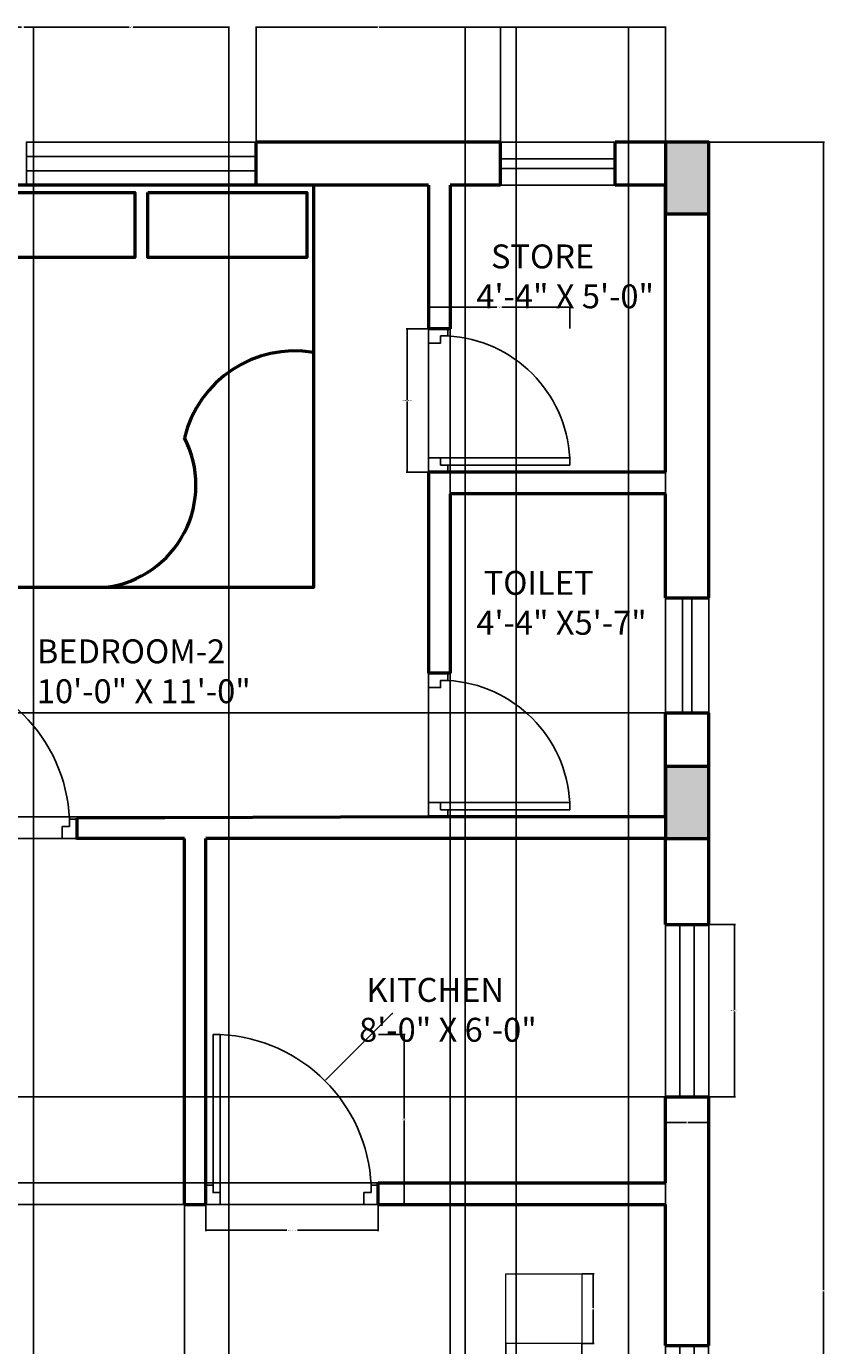
# Model space of a CAD drawing. Units: inches. Extents: x 2480 to 2840, y 795 to 1323.
# Tile 4 of 4: x 2673 to 2840, y 1047 to 1323. Entities that reach past the tile are written whole.
import ezdxf

# ---------------------------------------------------------------- set-up
doc = ezdxf.new("R2010")
doc.units = ezdxf.units.IN
for name, color, linetype, lineweight in [('A-ANNO-DIMS', 2, 'Continuous', 18), ('A-AREA-IDEN', 7, 'Continuous', 25), ('COLUMN', 240, 'Continuous', 50), ('door', 140, 'Continuous', 25), ('Furniture', 9, 'Continuous', 18), ('ventilator', 32, 'Continuous', 25), ('wall', 7, 'Continuous', 50), ('window', 201, 'Continuous', 25)]:
    doc.layers.add(name, color=color, linetype=linetype, lineweight=lineweight)
doc.styles.get("Standard").update_dxf_attribs({"font": 'arial.ttf'})
doc.dimstyles.get("Standard").update_dxf_attribs({"dimtxt": 0.18, "dimasz": 0.18, "dimexe": 0.18, "dimexo": 0.0625, "dimgap": 0.09, "dimtad": 0, "dimtih": 1, "dimtoh": 1, "dimdec": 4, "dimzin": 0, "dimdsep": 46, "dimtxsty": 'Standard', "dimcen": 0.09, "dimadec": 0, "dimazin": 0, "dimtfac": 1, "dimtdec": 4, "dimtofl": 0, "dimtmove": 0, "dimatfit": 3, "dimfxl": 1, "dimtolj": 1, "dimtzin": 0, "dimarcsym": 0})

# ---------------------------------------------------------------- blocks, each defined once
blk = doc.blocks.new('d1')
at = {"layer": 'door'}
blk.add_line((3049.73, 1052.02), (3085.73, 1052.02), dxfattribs=at)
blk.add_lwpolyline([(3051.23, 1054.52), (3052.73, 1054.52), (3052.73, 1087.52), (3051.23, 1087.52)], close=True, dxfattribs=at)
for points in [[(3052.73, 1052.02), (3049.73, 1052.02), (3049.73, 1056.02), (3051.23, 1056.02), (3051.23, 1054.52), (3052.73, 1054.52), (3052.73, 1052.02)], [(3082.73, 1052.02), (3085.73, 1052.02), (3085.73, 1056.02), (3084.23, 1056.02), (3084.23, 1054.52), (3082.73, 1054.52), (3082.73, 1052.02)]]:
    blk.add_lwpolyline(points, dxfattribs=at)
blk.add_arc((3051.23, 1054.52), 33.03, 2.6026, 87.3974, dxfattribs=at)
blk = doc.blocks.new('w2')
at = {"layer": 'window'}
for p, q in [((2880.46, 1137.77), (2880.46, 1101.77)), ((2883.46, 1137.77), (2883.46, 1101.77))]:
    blk.add_line(p, q, dxfattribs=at)
blk.add_lwpolyline([(2877.46, 1101.77), (2886.46, 1101.77), (2886.46, 1137.77), (2877.46, 1137.77)], close=True, dxfattribs=at)
blk = doc.blocks.new('v')
at = {"layer": 'ventilator'}
for p, q in [((2939.68, 1237.47), (2939.68, 1213.47)), ((2941.68, 1237.47), (2941.68, 1213.47))]:
    blk.add_line(p, q, dxfattribs=at)
blk.add_lwpolyline([(2936.18, 1213.47), (2945.18, 1213.47), (2945.18, 1237.47), (2936.18, 1237.47)], close=True, dxfattribs=at)
blk = doc.blocks.new('w1')
at = {"layer": 'window'}
for p, q in [((2922.2, 1100.57), (2922.2, 1052.57)), ((2925.2, 1100.57), (2925.2, 1052.57))]:
    blk.add_line(p, q, dxfattribs=at)
blk.add_lwpolyline([(2919.2, 1052.57), (2928.2, 1052.57), (2928.2, 1100.57), (2919.2, 1100.57)], close=True, dxfattribs=at)
blk = doc.blocks.new('d2')
at = {"layer": 'door'}
blk.add_line((3049.73, 993.24), (3079.73, 993.24), dxfattribs=at)
blk.add_lwpolyline([(3051.23, 995.74), (3052.73, 995.74), (3052.73, 1022.74), (3051.23, 1022.74)], close=True, dxfattribs=at)
for points in [[(3052.73, 993.24), (3049.73, 993.24), (3049.73, 997.24), (3051.23, 997.24), (3051.23, 995.74), (3052.73, 995.74), (3052.73, 993.24)], [(3076.73, 993.24), (3079.73, 993.24), (3079.73, 997.24), (3078.23, 997.24), (3078.23, 995.74), (3076.73, 995.74), (3076.73, 993.24)]]:
    blk.add_lwpolyline(points, dxfattribs=at)
blk.add_arc((3051.23, 995.74), 27.04, 3.1798, 86.8202, dxfattribs=at)
blk = doc.blocks.new('BED')
at = {"layer": 'wall'}
for points in [[(3037.98, 1220.47), (3109.98, 1220.47), (3109.98, 1304.47), (3037.98, 1304.47)], [(3039.4, 1302.95), (3072.6, 1302.95), (3072.6, 1289.33), (3039.4, 1289.33)], [(3075.32, 1302.95), (3108.52, 1302.95), (3108.52, 1289.33), (3075.32, 1289.33)]]:
    blk.add_lwpolyline(points, close=True, dxfattribs=at)
for centre, radius, start, end in [((3106.11, 1246.04), 23.81, 80.6483, 166.366), ((3063.91, 1241.76), 21.48, 277.4854, 27.4236)]:
    blk.add_arc(centre, radius, start, end, dxfattribs=at)
blk = doc.blocks.new('C')
at = {"layer": 'COLUMN'}
h = blk.add_hatch(color=256, dxfattribs=at)
h.dxf.hatch_style = 1
h.paths.add_polyline_path([(3016.24, 1218.72), (3031.24, 1218.72), (3031.24, 1227.72), (3016.24, 1227.72)])
blk.add_lwpolyline([(3016.24, 1218.72), (3031.24, 1218.72), (3031.24, 1227.72), (3016.24, 1227.72)], close=True, dxfattribs=at)
blk = doc.blocks.new('CHAIR-DINING')
blk.add_lwpolyline([(15.88, 0), (0, 0), (0, 14.61), (15.88, 14.61)], close=True)
blk = doc.blocks.new('*D14')
at = {"layer": 'A-ANNO-DIMS', "color": 0, "lineweight": -2, "transparency": 16777216}
for p, q in [((2816.02, 1135.24), (2821.53, 1135.24)), ((2821.35, 1135.06), (2821.35, 1117.42)), ((2821.35, 1099.42), (2821.35, 1117.06)), ((2816.02, 1099.24), (2821.53, 1099.24))]:
    blk.add_line(p, q, dxfattribs=at)
at = {"layer": 'A-ANNO-DIMS', "color": 0, "transparency": 16777216}
for points in [[(2821.32, 1135.06), (2821.38, 1135.06), (2821.35, 1135.24)], [(2821.32, 1099.42), (2821.38, 1099.42), (2821.35, 1099.24)]]:
    blk.add_solid(points, dxfattribs=at)
at = {"layer": 'Defpoints', "color": 0, "transparency": 16777216}
for p in [(2815.95, 1135.24), (2821.35, 1135.24), (2815.95, 1099.24)]:
    blk.add_point(p, dxfattribs=at)
at = {"layer": 'A-ANNO-DIMS', "color": 0, "transparency": 16777216, "insert": (2821.35, 1117.24), "char_height": 0.18, "attachment_point": 5}
blk.add_mtext('\\A1;WINDOW W2 36', dxfattribs=at)
blk = doc.blocks.new('*D15')
at = {"layer": 'A-ANNO-DIMS', "color": 0, "lineweight": -2, "transparency": 16777216}
for p, q in [((2806.95, 1099.18), (2806.95, 1093.66)), ((2815.95, 1099.18), (2815.95, 1093.66)), ((2807.13, 1093.84), (2811.3, 1093.84)), ((2815.77, 1093.84), (2811.6, 1093.84))]:
    blk.add_line(p, q, dxfattribs=at)
at = {"layer": 'A-ANNO-DIMS', "color": 0, "transparency": 16777216}
for points in [[(2807.13, 1093.87), (2807.13, 1093.81), (2806.95, 1093.84)], [(2815.77, 1093.87), (2815.77, 1093.81), (2815.95, 1093.84)]]:
    blk.add_solid(points, dxfattribs=at)
at = {"layer": 'Defpoints', "color": 0, "transparency": 16777216}
for p in [(2806.95, 1099.24), (2815.95, 1099.24), (2815.95, 1093.84)]:
    blk.add_point(p, dxfattribs=at)
at = {"layer": 'A-ANNO-DIMS', "color": 0, "transparency": 16777216, "insert": (2811.45, 1093.84), "char_height": 0.18, "attachment_point": 5}
blk.add_mtext('\\A1;9', dxfattribs=at)
blk = doc.blocks.new('*D18')
at = {"layer": 'A-ANNO-DIMS', "color": 0, "lineweight": -2, "transparency": 16777216}
for p, q in [((2710.95, 1076.68), (2710.95, 1071.16)), ((2746.95, 1076.68), (2746.95, 1071.16)), ((2711.13, 1071.34), (2727.82, 1071.34)), ((2746.77, 1071.34), (2730.08, 1071.34))]:
    blk.add_line(p, q, dxfattribs=at)
at = {"layer": 'A-ANNO-DIMS', "color": 0, "transparency": 16777216}
for points in [[(2711.13, 1071.37), (2711.13, 1071.31), (2710.95, 1071.34)], [(2746.77, 1071.37), (2746.77, 1071.31), (2746.95, 1071.34)]]:
    blk.add_solid(points, dxfattribs=at)
at = {"layer": 'Defpoints', "color": 0, "transparency": 16777216}
for p in [(2710.95, 1076.74), (2746.95, 1076.74), (2746.95, 1071.34)]:
    blk.add_point(p, dxfattribs=at)
at = {"layer": 'A-ANNO-DIMS', "color": 0, "transparency": 16777216, "insert": (2728.95, 1071.34), "char_height": 0.18, "attachment_point": 5}
blk.add_mtext('\\A1;DOOR D1 36 TYP.', dxfattribs=at)
blk = doc.blocks.new('*D19')
at = {"layer": 'A-ANNO-DIMS', "color": 0, "lineweight": -2, "transparency": 16777216}
for p, q in [((2747.02, 1112.24), (2752.53, 1112.24)), ((2752.35, 1112.06), (2752.35, 1094.67)), ((2752.35, 1076.92), (2752.35, 1094.31)), ((2747.02, 1076.74), (2752.53, 1076.74))]:
    blk.add_line(p, q, dxfattribs=at)
at = {"layer": 'A-ANNO-DIMS', "color": 0, "transparency": 16777216}
for points in [[(2752.32, 1112.06), (2752.38, 1112.06), (2752.35, 1112.24)], [(2752.32, 1076.92), (2752.38, 1076.92), (2752.35, 1076.74)]]:
    blk.add_solid(points, dxfattribs=at)
at = {"layer": 'Defpoints', "color": 0, "transparency": 16777216}
for p in [(2746.95, 1112.24), (2752.35, 1112.24), (2746.95, 1076.74)]:
    blk.add_point(p, dxfattribs=at)
at = {"layer": 'A-ANNO-DIMS', "color": 0, "transparency": 16777216, "insert": (2752.35, 1094.49), "char_height": 0.18, "attachment_point": 5}
blk.add_mtext('\\A1;36 TYP.', dxfattribs=at)
blk = doc.blocks.new('*D20')
at = {"layer": 'A-ANNO-DIMS', "color": 0, "lineweight": -2, "transparency": 16777216}
for p, q in [((2757.39, 1259.74), (2752.77, 1259.74)), ((2752.95, 1259.56), (2752.95, 1244.92)), ((2752.95, 1229.92), (2752.95, 1244.56)), ((2757.39, 1229.74), (2752.77, 1229.74))]:
    blk.add_line(p, q, dxfattribs=at)
at = {"layer": 'A-ANNO-DIMS', "color": 0, "transparency": 16777216}
for points in [[(2752.92, 1259.56), (2752.98, 1259.56), (2752.95, 1259.74)], [(2752.92, 1229.92), (2752.98, 1229.92), (2752.95, 1229.74)]]:
    blk.add_solid(points, dxfattribs=at)
at = {"layer": 'Defpoints', "color": 0, "transparency": 16777216}
for p in [(2752.95, 1259.74), (2757.45, 1259.74), (2757.45, 1229.74)]:
    blk.add_point(p, dxfattribs=at)
at = {"layer": 'A-ANNO-DIMS', "color": 0, "transparency": 16777216, "insert": (2752.95, 1244.74), "char_height": 0.18, "attachment_point": 5}
blk.add_mtext('\\A1;DOOR D2 30 TYP.', dxfattribs=at)
blk = doc.blocks.new('*D21')
at = {"layer": 'A-ANNO-DIMS', "color": 0, "lineweight": -2, "transparency": 16777216}
for p, q in [((2757.45, 1259.8), (2757.45, 1264.42)), ((2757.63, 1264.24), (2771.68, 1264.24)), ((2786.77, 1264.24), (2772.73, 1264.24)), ((2786.95, 1259.8), (2786.95, 1264.42))]:
    blk.add_line(p, q, dxfattribs=at)
at = {"layer": 'A-ANNO-DIMS', "color": 0, "transparency": 16777216}
for points in [[(2757.63, 1264.27), (2757.63, 1264.21), (2757.45, 1264.24)], [(2786.77, 1264.27), (2786.77, 1264.21), (2786.95, 1264.24)]]:
    blk.add_solid(points, dxfattribs=at)
at = {"layer": 'Defpoints', "color": 0, "transparency": 16777216}
for p in [(2786.95, 1264.24), (2757.45, 1259.74), (2786.95, 1259.74)]:
    blk.add_point(p, dxfattribs=at)
at = {"layer": 'A-ANNO-DIMS', "color": 0, "transparency": 16777216, "insert": (2772.2, 1264.24), "char_height": 0.18, "attachment_point": 5}
blk.add_mtext('\\A1;30 TYP.', dxfattribs=at)
blk = doc.blocks.new('*D26')
at = {"layer": 'A-ANNO-DIMS', "color": 0, "lineweight": -2, "transparency": 16777216}
for p, q in [((2773.57, 1047.6), (2773.57, 1045.1)), ((2773.75, 1045.28), (2780.09, 1045.28)), ((2789.27, 1045.28), (2782.94, 1045.28)), ((2789.45, 1047.6), (2789.45, 1045.1))]:
    blk.add_line(p, q, dxfattribs=at)
at = {"layer": 'A-ANNO-DIMS', "color": 0, "transparency": 16777216}
for points in [[(2773.75, 1045.31), (2773.75, 1045.25), (2773.57, 1045.28)], [(2789.27, 1045.31), (2789.27, 1045.25), (2789.45, 1045.28)]]:
    blk.add_solid(points, dxfattribs=at)
at = {"layer": 'Defpoints', "color": 0, "transparency": 16777216}
for p in [(2773.57, 1047.66), (2789.45, 1047.66), (2789.45, 1045.28)]:
    blk.add_point(p, dxfattribs=at)
at = {"layer": 'A-ANNO-DIMS', "color": 0, "transparency": 16777216, "insert": (2781.51, 1045.28), "char_height": 0.18, "attachment_point": 5}
blk.add_mtext('\\A1;DINING CHAIR 16 TYP.', dxfattribs=at)
blk = doc.blocks.new('*D27')
at = {"layer": 'A-ANNO-DIMS', "color": 0, "lineweight": -2, "transparency": 16777216}
for p, q in [((2789.52, 1062.27), (2792.02, 1062.27)), ((2791.84, 1062.09), (2791.84, 1055.15)), ((2791.84, 1047.84), (2791.84, 1054.78)), ((2789.52, 1047.66), (2792.02, 1047.66))]:
    blk.add_line(p, q, dxfattribs=at)
at = {"layer": 'A-ANNO-DIMS', "color": 0, "transparency": 16777216}
for points in [[(2791.81, 1062.09), (2791.87, 1062.09), (2791.84, 1062.27)], [(2791.81, 1047.84), (2791.87, 1047.84), (2791.84, 1047.66)]]:
    blk.add_solid(points, dxfattribs=at)
at = {"layer": 'Defpoints', "color": 0, "transparency": 16777216}
for p in [(2789.45, 1062.27), (2791.84, 1062.27), (2789.45, 1047.66)]:
    blk.add_point(p, dxfattribs=at)
at = {"layer": 'A-ANNO-DIMS', "color": 0, "transparency": 16777216, "insert": (2791.84, 1054.96), "char_height": 0.18, "attachment_point": 5}
blk.add_mtext('\\A1;15 TYP.', dxfattribs=at)
blk = doc.blocks.new('*D29')
at = {"layer": 'A-ANNO-DIMS', "color": 0, "lineweight": -2, "transparency": 16777216}
for p, q in [((2816.02, 1298.74), (2840.14, 1298.74)), ((2839.96, 1298.56), (2839.96, 1058.92)), ((2839.96, 818.92), (2839.96, 1058.56)), ((2816.02, 818.74), (2840.14, 818.74))]:
    blk.add_line(p, q, dxfattribs=at)
at = {"layer": 'A-ANNO-DIMS', "color": 0, "transparency": 16777216}
for points in [[(2839.93, 1298.56), (2839.99, 1298.56), (2839.96, 1298.74)], [(2839.93, 818.92), (2839.99, 818.92), (2839.96, 818.74)]]:
    blk.add_solid(points, dxfattribs=at)
at = {"layer": 'Defpoints', "color": 0, "transparency": 16777216}
for p in [(2815.95, 1298.74), (2839.96, 1298.74), (2815.95, 818.74)]:
    blk.add_point(p, dxfattribs=at)
at = {"layer": 'A-ANNO-DIMS', "color": 0, "transparency": 16777216, "insert": (2839.96, 1058.74), "char_height": 0.18, "attachment_point": 5}
blk.add_mtext('\\A1;480', dxfattribs=at)
blk = doc.blocks.new('*D32')
at = {"layer": 'A-ANNO-DIMS', "color": 0, "lineweight": -2, "transparency": 16777216}
for p, q in [((2721.45, 1298.8), (2721.45, 1322.93)), ((2721.63, 1322.75), (2746.75, 1322.75)), ((2772.27, 1322.75), (2747.16, 1322.75)), ((2772.45, 1298.8), (2772.45, 1322.93))]:
    blk.add_line(p, q, dxfattribs=at)
at = {"layer": 'A-ANNO-DIMS', "color": 0, "transparency": 16777216}
for points in [[(2721.63, 1322.78), (2721.63, 1322.72), (2721.45, 1322.75)], [(2772.27, 1322.78), (2772.27, 1322.72), (2772.45, 1322.75)]]:
    blk.add_solid(points, dxfattribs=at)
at = {"layer": 'Defpoints', "color": 0, "transparency": 16777216}
for p in [(2772.45, 1322.75), (2721.45, 1298.74), (2772.45, 1298.74)]:
    blk.add_point(p, dxfattribs=at)
at = {"layer": 'A-ANNO-DIMS', "color": 0, "transparency": 16777216, "insert": (2746.95, 1322.75), "char_height": 0.18, "attachment_point": 5}
blk.add_mtext('\\A1;51', dxfattribs=at)
blk = doc.blocks.new('*D39')
at = {"layer": 'A-ANNO-DIMS', "color": 0, "lineweight": -2, "transparency": 16777216}
for p, q in [((2806.89, 1099.24), (2479.77, 1099.24)), ((2479.95, 1099.06), (2479.95, 1090.42)), ((2479.95, 1081.42), (2479.95, 1090.06)), ((2806.89, 1081.24), (2479.77, 1081.24))]:
    blk.add_line(p, q, dxfattribs=at)
at = {"layer": 'A-ANNO-DIMS', "color": 0, "transparency": 16777216}
for points in [[(2479.92, 1099.06), (2479.98, 1099.06), (2479.95, 1099.24)], [(2479.92, 1081.42), (2479.98, 1081.42), (2479.95, 1081.24)]]:
    blk.add_solid(points, dxfattribs=at)
at = {"layer": 'Defpoints', "color": 0, "transparency": 16777216}
for p in [(2479.95, 1099.24), (2806.95, 1099.24), (2806.95, 1081.24)]:
    blk.add_point(p, dxfattribs=at)
at = {"layer": 'A-ANNO-DIMS', "color": 0, "transparency": 16777216, "insert": (2479.95, 1090.24), "char_height": 0.18, "attachment_point": 5}
blk.add_mtext('\\A1;18', dxfattribs=at)
blk = doc.blocks.new('*D40')
at = {"layer": 'A-ANNO-DIMS', "color": 0, "lineweight": -2, "transparency": 16777216}
for p, q in [((2806.89, 1179.49), (2479.77, 1179.49)), ((2479.95, 1179.31), (2479.95, 1168.8)), ((2479.95, 1157.92), (2479.95, 1168.43)), ((2806.89, 1157.74), (2479.77, 1157.74))]:
    blk.add_line(p, q, dxfattribs=at)
at = {"layer": 'A-ANNO-DIMS', "color": 0, "transparency": 16777216}
for points in [[(2479.92, 1179.31), (2479.98, 1179.31), (2479.95, 1179.49)], [(2479.92, 1157.92), (2479.98, 1157.92), (2479.95, 1157.74)]]:
    blk.add_solid(points, dxfattribs=at)
at = {"layer": 'Defpoints', "color": 0, "transparency": 16777216}
for p in [(2479.95, 1179.49), (2806.95, 1179.49), (2806.95, 1157.74)]:
    blk.add_point(p, dxfattribs=at)
at = {"layer": 'A-ANNO-DIMS', "color": 0, "transparency": 16777216, "insert": (2479.95, 1168.62), "char_height": 0.18, "attachment_point": 5}
blk.add_mtext('\\A1;21.75', dxfattribs=at)
blk = doc.blocks.new('*D41')
at = {"layer": 'A-ANNO-DIMS', "color": 0, "lineweight": -2, "transparency": 16777216}
for p, q in [((2775.71, 827.8), (2775.71, 1322.93)), ((2775.89, 1322.75), (2790.94, 1322.75)), ((2806.77, 1322.75), (2791.73, 1322.75)), ((2806.95, 827.8), (2806.95, 1322.93))]:
    blk.add_line(p, q, dxfattribs=at)
at = {"layer": 'A-ANNO-DIMS', "color": 0, "transparency": 16777216}
for points in [[(2775.89, 1322.78), (2775.89, 1322.72), (2775.71, 1322.75)], [(2806.77, 1322.78), (2806.77, 1322.72), (2806.95, 1322.75)]]:
    blk.add_solid(points, dxfattribs=at)
at = {"layer": 'Defpoints', "color": 0, "transparency": 16777216}
for p in [(2806.95, 1322.75), (2775.71, 827.74), (2806.95, 827.74)]:
    blk.add_point(p, dxfattribs=at)
at = {"layer": 'A-ANNO-DIMS', "color": 0, "transparency": 16777216, "insert": (2791.33, 1322.75), "char_height": 0.18, "attachment_point": 5}
blk.add_mtext('\\A1;31.24', dxfattribs=at)
blk = doc.blocks.new('*D44')
at = {"layer": 'A-ANNO-DIMS', "color": 0, "lineweight": -2, "transparency": 16777216}
for p, q in [((2706.39, 1076.74), (2479.77, 1076.74)), ((2479.95, 1076.56), (2479.95, 1023.42)), ((2479.95, 969.92), (2479.95, 1023.06)), ((2710.89, 969.74), (2479.77, 969.74))]:
    blk.add_line(p, q, dxfattribs=at)
at = {"layer": 'A-ANNO-DIMS', "color": 0, "transparency": 16777216}
for points in [[(2479.92, 1076.56), (2479.98, 1076.56), (2479.95, 1076.74)], [(2479.92, 969.92), (2479.98, 969.92), (2479.95, 969.74)]]:
    blk.add_solid(points, dxfattribs=at)
at = {"layer": 'Defpoints', "color": 0, "transparency": 16777216}
for p in [(2479.95, 1076.74), (2706.45, 1076.74), (2710.95, 969.74)]:
    blk.add_point(p, dxfattribs=at)
at = {"layer": 'A-ANNO-DIMS', "color": 0, "transparency": 16777216, "insert": (2479.95, 1023.24), "char_height": 0.18, "attachment_point": 5}
blk.add_mtext('\\A1;107', dxfattribs=at)
blk = doc.blocks.new('*D50')
at = {"layer": 'A-ANNO-DIMS', "color": 0, "lineweight": -2, "transparency": 16777216}
for p, q in [((2637.45, 1076.68), (2637.45, 794.56)), ((2706.45, 1076.68), (2706.45, 794.56)), ((2637.63, 794.74), (2671.73, 794.74)), ((2706.27, 794.74), (2672.17, 794.74))]:
    blk.add_line(p, q, dxfattribs=at)
at = {"layer": 'A-ANNO-DIMS', "color": 0, "transparency": 16777216}
for points in [[(2637.63, 794.77), (2637.63, 794.71), (2637.45, 794.74)], [(2706.27, 794.77), (2706.27, 794.71), (2706.45, 794.74)]]:
    blk.add_solid(points, dxfattribs=at)
at = {"layer": 'Defpoints', "color": 0, "transparency": 16777216}
for p in [(2637.45, 1076.74), (2706.45, 1076.74), (2706.45, 794.74)]:
    blk.add_point(p, dxfattribs=at)
at = {"layer": 'A-ANNO-DIMS', "color": 0, "transparency": 16777216, "insert": (2671.95, 794.74), "char_height": 0.18, "attachment_point": 5}
blk.add_mtext('\\A1;69', dxfattribs=at)
blk = doc.blocks.new('*D51')
at = {"layer": 'A-ANNO-DIMS', "color": 0, "lineweight": -2, "transparency": 16777216}
for p, q in [((2761.95, 1289.68), (2761.95, 794.56)), ((2806.95, 1289.68), (2806.95, 794.56)), ((2762.13, 794.74), (2784.23, 794.74)), ((2806.77, 794.74), (2784.68, 794.74))]:
    blk.add_line(p, q, dxfattribs=at)
at = {"layer": 'A-ANNO-DIMS', "color": 0, "transparency": 16777216}
for points in [[(2762.13, 794.77), (2762.13, 794.71), (2761.95, 794.74)], [(2806.77, 794.77), (2806.77, 794.71), (2806.95, 794.74)]]:
    blk.add_solid(points, dxfattribs=at)
at = {"layer": 'Defpoints', "color": 0, "transparency": 16777216}
for p in [(2761.95, 1289.74), (2806.95, 1289.74), (2806.95, 794.74)]:
    blk.add_point(p, dxfattribs=at)
at = {"layer": 'A-ANNO-DIMS', "color": 0, "transparency": 16777216, "insert": (2784.45, 794.74), "char_height": 0.18, "attachment_point": 5}
blk.add_mtext('\\A1;45', dxfattribs=at)
blk = doc.blocks.new('*D52')
at = {"layer": 'A-ANNO-DIMS', "color": 0, "lineweight": -2, "transparency": 16777216}
for p, q in [((2670.45, 818.8), (2670.45, 1322.93)), ((2670.63, 1322.75), (2672.45, 1322.75)), ((2674.77, 1322.75), (2672.96, 1322.75)), ((2674.95, 827.8), (2674.95, 1322.93))]:
    blk.add_line(p, q, dxfattribs=at)
at = {"layer": 'A-ANNO-DIMS', "color": 0, "transparency": 16777216}
for points in [[(2670.63, 1322.78), (2670.63, 1322.72), (2670.45, 1322.75)], [(2674.77, 1322.78), (2674.77, 1322.72), (2674.95, 1322.75)]]:
    blk.add_solid(points, dxfattribs=at)
at = {"layer": 'Defpoints', "color": 0, "transparency": 16777216}
for p in [(2674.95, 1322.75), (2674.95, 827.74), (2670.45, 818.74)]:
    blk.add_point(p, dxfattribs=at)
at = {"layer": 'A-ANNO-DIMS', "color": 0, "transparency": 16777216, "insert": (2672.7, 1322.75), "char_height": 0.18, "attachment_point": 5}
blk.add_mtext('\\A1;4.5', dxfattribs=at)
blk = doc.blocks.new('*D57')
at = {"layer": 'A-ANNO-DIMS', "color": 0, "lineweight": -2, "transparency": 16777216}
for p, q in [((2765.09, 995.24), (2765.09, 1322.93)), ((2765.27, 1322.75), (2781.68, 1322.75)), ((2799.02, 1322.75), (2782.61, 1322.75)), ((2799.2, 995.24), (2799.2, 1322.93))]:
    blk.add_line(p, q, dxfattribs=at)
at = {"layer": 'A-ANNO-DIMS', "color": 0, "transparency": 16777216}
for points in [[(2765.27, 1322.78), (2765.27, 1322.72), (2765.09, 1322.75)], [(2799.02, 1322.78), (2799.02, 1322.72), (2799.2, 1322.75)]]:
    blk.add_solid(points, dxfattribs=at)
at = {"layer": 'Defpoints', "color": 0, "transparency": 16777216}
for p in [(2799.2, 1322.75), (2765.09, 995.18), (2799.2, 995.18)]:
    blk.add_point(p, dxfattribs=at)
at = {"layer": 'A-ANNO-DIMS', "color": 0, "transparency": 16777216, "insert": (2782.14, 1322.75), "char_height": 0.18, "attachment_point": 5}
blk.add_mtext('\\A1;34.114', dxfattribs=at)
blk = doc.blocks.new('*D61')
at = {"layer": 'A-ANNO-DIMS', "color": 0, "lineweight": -2, "transparency": 16777216}
for p, q in [((2799.2, 1044.3), (2799.2, 1322.93)), ((2799.38, 1322.75), (2802.69, 1322.75)), ((2806.77, 1322.75), (2803.47, 1322.75)), ((2806.95, 1047.3), (2806.95, 1322.93))]:
    blk.add_line(p, q, dxfattribs=at)
at = {"layer": 'A-ANNO-DIMS', "color": 0, "transparency": 16777216}
for points in [[(2799.38, 1322.78), (2799.38, 1322.72), (2799.2, 1322.75)], [(2806.77, 1322.78), (2806.77, 1322.72), (2806.95, 1322.75)]]:
    blk.add_solid(points, dxfattribs=at)
at = {"layer": 'Defpoints', "color": 0, "transparency": 16777216}
for p in [(2799.2, 1322.75), (2806.95, 1047.24), (2799.2, 1044.23)]:
    blk.add_point(p, dxfattribs=at)
at = {"layer": 'A-ANNO-DIMS', "color": 0, "transparency": 16777216, "insert": (2803.08, 1322.75), "char_height": 0.18, "attachment_point": 5}
blk.add_mtext('\\A1;7.752', dxfattribs=at)
blk = doc.blocks.new('*D67')
at = {"layer": 'A-ANNO-DIMS', "color": 0, "lineweight": -2, "transparency": 16777216}
for p, q in [((2674.95, 827.8), (2674.95, 1322.93)), ((2675.13, 1322.75), (2694.94, 1322.75)), ((2715.53, 1322.75), (2695.73, 1322.75)), ((2715.71, 827.8), (2715.71, 1322.93))]:
    blk.add_line(p, q, dxfattribs=at)
at = {"layer": 'A-ANNO-DIMS', "color": 0, "transparency": 16777216}
for points in [[(2675.13, 1322.78), (2675.13, 1322.72), (2674.95, 1322.75)], [(2715.53, 1322.78), (2715.53, 1322.72), (2715.71, 1322.75)]]:
    blk.add_solid(points, dxfattribs=at)
at = {"layer": 'Defpoints', "color": 0, "transparency": 16777216}
for p in [(2715.71, 1322.75), (2674.95, 827.74), (2715.71, 827.74)]:
    blk.add_point(p, dxfattribs=at)
at = {"layer": 'A-ANNO-DIMS', "color": 0, "transparency": 16777216, "insert": (2695.33, 1322.75), "char_height": 0.18, "attachment_point": 5}
blk.add_mtext('\\A1;40.76', dxfattribs=at)
blk = doc.blocks.new('*D69')
at = {"layer": 'A-ANNO-DIMS', "color": 0, "lineweight": -2, "transparency": 16777216}
for p, q in [((2749.83, 1116.62), (2735.94, 1102.73)), ((2750.01, 1116.62), (2749.83, 1116.62)), ((2712.36, 1079.24), (2712.54, 1079.24)), ((2712.45, 1079.15), (2712.45, 1079.33))]:
    blk.add_line(p, q, dxfattribs=at)
at = {"layer": 'A-ANNO-DIMS', "color": 0, "transparency": 16777216}
blk.add_solid([(2735.92, 1102.75), (2735.96, 1102.71), (2735.81, 1102.6)], dxfattribs=at)
at = {"layer": 'Defpoints', "color": 0, "transparency": 16777216}
for p in [(2735.81, 1102.6), (2712.45, 1079.24)]:
    blk.add_point(p, dxfattribs=at)
at = {"layer": 'A-ANNO-DIMS', "color": 0, "transparency": 16777216, "insert": (2750.75, 1116.62), "char_height": 0.18, "attachment_point": 5}
blk.add_mtext('\\A1;4X R33.034', dxfattribs=at)

msp = doc.modelspace()

# ---------------------------------------------------------------- linework, layer by layer
at = {"layer": 'wall'}
for p, q in [((2721.4535, 1289.7416), (2721.4535, 1298.7416)), ((2772.4535, 1298.7416), (2721.4535, 1298.7416)), ((2772.4535, 1289.7416), (2772.4535, 1298.7416)), ((2815.9535, 1298.7416), (2796.4535, 1298.7416)), ((2796.4535, 1289.7416), (2796.4535, 1298.7416)), ((2815.9535, 1203.4916), (2815.9535, 1298.7416)), ((2757.4535, 1289.7416), (2721.4535, 1289.7416)), ((2757.4535, 1289.7416), (2757.4535, 1259.7416)), ((2761.9535, 1289.7416), (2761.9535, 1259.7416)), ((2772.4535, 1289.7416), (2761.9535, 1289.7416)), ((2806.9535, 1289.7416), (2796.4535, 1289.7416)), ((2806.9535, 1229.7416), (2806.9535, 1289.7416)), ((2761.9535, 1259.7416), (2757.4535, 1259.7416)), ((2806.9535, 1229.7416), (2757.4535, 1229.7416)), ((2757.4535, 1229.7416), (2757.4535, 1187.7416)), ((2806.9535, 1225.2416), (2761.9535, 1225.2416)), ((2761.9535, 1225.2416), (2761.9535, 1187.7416)), ((2806.9535, 1203.4916), (2806.9535, 1225.2416)), ((2806.9535, 1203.4916), (2815.9535, 1203.4916)), ((2761.9535, 1187.7416), (2757.4535, 1187.7416)), ((2806.9535, 1157.7416), (2806.9535, 1179.4916)), ((2806.9535, 1179.4916), (2815.9535, 1179.4916)), ((2815.9535, 1135.2416), (2815.9535, 1179.4916)), ((2757.4535, 1157.7416), (2683.9535, 1157.4916)), ((2683.9535, 1157.4916), (2683.9535, 1152.9916)), ((2806.9535, 1157.7416), (2757.4535, 1157.7416)), ((2706.4535, 1153.2416), (2683.9535, 1153.2416)), ((2706.4535, 1076.7416), (2706.4535, 1153.2416)), ((2806.9535, 1153.2416), (2710.9535, 1153.2416)), ((2710.9535, 1076.7416), (2710.9535, 1153.2416)), ((2806.9535, 1135.2416), (2806.9535, 1153.2416)), ((2806.9535, 1135.2416), (2815.9535, 1135.2416)), ((2806.9535, 1081.2416), (2806.9535, 1099.2416)), ((2806.9535, 1099.2416), (2815.9535, 1099.2416)), ((2815.9535, 1047.2416), (2815.9535, 1099.2416)), ((2746.9535, 1081.2416), (2806.9535, 1081.2416)), ((2746.9535, 1076.7416), (2746.9535, 1081.2416)), ((2706.4535, 1076.7416), (2710.9535, 1076.7416)), ((2746.9535, 1076.7416), (2806.9535, 1076.7416)), ((2806.9535, 1047.2416), (2806.9535, 1076.7416)), ((2806.9535, 1047.2416), (2815.9535, 1047.2416))]:
    msp.add_line(p, q, dxfattribs=at)

# ---------------------------------------------------------------- block references
at = {"layer": 'COLUMN', "rotation": 270}
for p in [(1588.2303, 4314.9817), (1588.2303, 4184.4817)]:
    msp.add_blockref('C', p, dxfattribs=at)
at = {"layer": 'door', "xscale": -1, "rotation": 270}
for p in [(1764.2101, -1819.9908), (1764.2101, -1891.9908)]:
    msp.add_blockref('d2', p, dxfattribs=at)
at = {"layer": 'door'}
for p in [(-401.7789, 101.2216), (-338.7789, 24.7216)]:
    msp.add_blockref('d1', p, dxfattribs=at)
at = {"layer": 'Furniture'}
for name, p in [('BED', (-376.525, -14.7245)), ('CHAIR-DINING', (2773.571, 1047.659))]:
    msp.add_blockref(name, p, dxfattribs=at)
at = {"layer": 'ventilator', "rotation": 270}
msp.add_blockref('v', (1558.9818, 4234.9217), dxfattribs=at)
at = {"layer": 'ventilator'}
msp.add_blockref('v', (-129.2266, -33.9801), dxfattribs=at)
at = {"layer": 'window', "rotation": 90}
msp.add_blockref('w1', (3774.0221, -1629.4626), dxfattribs=at)
at = {"layer": 'window'}
for name, p in [('w2', (-70.506, -2.5237)), ('w1', (-112.2506, -53.327))]:
    msp.add_blockref(name, p, dxfattribs=at)

# ---------------------------------------------------------------- texts
at = {"layer": 'A-AREA-IDEN', "char_height": 5, "attachment_point": 1}
for s, insert in [('  STORE\\P4\'-4" X 5\'-0"', (2767.4309, 1277.354)), (' TOILET\\P4\'-4" X5\'-7"', (2767.4309, 1209.1361)), ('BEDROOM-2\\P10\'-0" X 11\'-0"', (2675.6401, 1194.8303)), (' KITCHEN\\P8\'-0" X 6\'-0"', (2742.9393, 1124.0771))]:
    msp.add_mtext_dynamic_manual_height_columns(s, width=47.7919, gutter_width=12.5, heights=[0], dxfattribs=dict(at, insert=insert))

# ---------------------------------------------------------------- dimensions: what is measured, and where the dimension line sits
at = {"layer": 'A-ANNO-DIMS'}
for base, p1, p2, override, picture, middle in [((2674.9535, 1322.7466), (2670.4535, 818.7416), (2674.9535, 827.7416), {"dimdec": 1, "dimlfac": 1, "dimrnd": 0, "dimzin": 0, "dimdsep": 46, "dimlunit": 2}, '*D52', (2672.7035, 1322.7466)), ((2715.7148, 1322.7466), (2674.9535, 827.7416), (2715.7148, 827.7416), {"dimdec": 2, "dimlfac": 1, "dimrnd": 0, "dimzin": 0, "dimdsep": 46, "dimlunit": 2}, '*D67', (2695.3342, 1322.7466)), ((2772.4535, 1322.7466), (2721.4535, 1298.7416), (2772.4535, 1298.7416), {"dimdec": 0, "dimlfac": 1, "dimrnd": 0, "dimzin": 0, "dimdsep": 46, "dimlunit": 2}, '*D32', (2746.9535, 1322.7466)), ((2799.2019, 1322.7466), (2765.0875, 995.1772), (2799.2019, 995.1772), {"dimdec": 3, "dimlfac": 1, "dimrnd": 0, "dimzin": 0, "dimdsep": 46, "dimlunit": 2}, '*D57', (2782.1447, 1322.7466)), ((2806.9535, 1322.7466), (2775.7148, 827.7416), (2806.9535, 827.7416), {"dimdec": 2, "dimlfac": 1, "dimrnd": 0, "dimzin": 0, "dimdsep": 46, "dimlunit": 2}, '*D41', (2791.3342, 1322.7466)), ((2799.2019, 1322.7466), (2806.9535, 1047.2416), (2799.2019, 1044.2327), {"dimdec": 3, "dimlfac": 1, "dimrnd": 0, "dimzin": 0, "dimdsep": 46, "dimlunit": 2}, '*D61', (2803.0777, 1322.7466)), ((2806.9535, 794.7366), (2761.9535, 1289.7416), (2806.9535, 1289.7416), {"dimdec": 0, "dimlfac": 1, "dimrnd": 0, "dimzin": 0, "dimdsep": 46, "dimlunit": 2}, '*D51', (2784.4535, 794.7366)), ((2815.9535, 1093.8416), (2806.9535, 1099.2416), (2815.9535, 1099.2416), {"dimdec": 0, "dimlfac": 1, "dimrnd": 0, "dimzin": 0, "dimdsep": 46, "dimlunit": 2}, '*D15', (2811.4535, 1093.8416)), ((2706.4535, 794.7366), (2637.4535, 1076.7416), (2706.4535, 1076.7416), {"dimdec": 0, "dimlfac": 1, "dimrnd": 0, "dimzin": 0, "dimdsep": 46, "dimlunit": 2}, '*D50', (2671.9535, 794.7366))]:
    dim = msp.add_linear_dim(base=base, p1=p1, p2=p2, dimstyle='Standard', override=override, dxfattribs=at)
    dim.commit()
    dim.dimension.update_dxf_attribs({"geometry": picture, "text_midpoint": middle})
for base, p1, p2, override, picture, middle in [((2839.9585, 1298.7416), (2815.9535, 818.7416), (2815.9535, 1298.7416), {"dimdec": 0, "dimlfac": 1, "dimrnd": 0, "dimzin": 0, "dimdsep": 46, "dimlunit": 2}, '*D29', (2839.9585, 1058.7416)), ((2479.9485, 1179.4916), (2806.9535, 1157.7416), (2806.9535, 1179.4916), {"dimdec": 2, "dimlfac": 1, "dimrnd": 0, "dimzin": 0, "dimdsep": 46, "dimlunit": 2}, '*D40', (2479.9485, 1168.6166)), ((2479.9485, 1099.2416), (2806.9535, 1081.2416), (2806.9535, 1099.2416), {"dimdec": 0, "dimlfac": 1, "dimrnd": 0, "dimzin": 0, "dimdsep": 46, "dimlunit": 2}, '*D39', (2479.9485, 1090.2416)), ((2479.9485, 1076.7416), (2710.9535, 969.7416), (2706.4535, 1076.7416), {"dimdec": 0, "dimlfac": 1, "dimrnd": 0, "dimzin": 0, "dimdsep": 46, "dimlunit": 2}, '*D44', (2479.9485, 1023.2416))]:
    dim = msp.add_linear_dim(base=base, p1=p1, p2=p2, angle=90, dimstyle='Standard', override=override, dxfattribs=at)
    dim.commit()
    dim.dimension.update_dxf_attribs({"geometry": picture, "text_midpoint": middle})
for base, p1, p2, text, picture, middle in [((2786.9535254586, 1264.241590311), (2757.4535254586, 1259.741590311), (2786.9535254586, 1259.741590311), '<> TYP.', '*D21', (2772.2035254586, 1264.241590311)), ((2746.9535, 1071.3416), (2710.9535, 1076.7416), (2746.9535, 1076.7416), 'DOOR D1 <> TYP.', '*D18', (2728.9535, 1071.3416)), ((2789.4549, 1045.2768), (2773.571, 1047.6594), (2789.4549, 1047.6594), 'DINING CHAIR <> TYP.', '*D26', (2781.513, 1045.2768))]:
    dim = msp.add_linear_dim(base=base, p1=p1, p2=p2, text=text, dimstyle='Standard', override={"dimdec": 0, "dimlfac": 1, "dimrnd": 0, "dimzin": 0, "dimdsep": 46, "dimlunit": 2}, dxfattribs=at)
    dim.commit()
    dim.dimension.update_dxf_attribs({"geometry": picture, "text_midpoint": middle})
for base, p1, p2, text, picture, middle in [((2752.9535, 1259.7416), (2757.4535, 1229.7416), (2757.4535, 1259.7416), 'DOOR D2 <> TYP.', '*D20', (2752.9535, 1244.7416)), ((2821.3535, 1135.2416), (2815.9535, 1099.2416), (2815.9535, 1135.2416), 'WINDOW W2 <>', '*D14', (2821.3535, 1117.2416)), ((2752.3535254586, 1112.241590311), (2746.9535254586, 1076.741590311), (2746.9535254586, 1112.241590311), '<> TYP.', '*D19', (2752.3535254586, 1094.491590311)), ((2791.8375, 1062.2678), (2789.4549, 1047.6594), (2789.4549, 1062.2678), '<> TYP.', '*D27', (2791.8375, 1054.9636))]:
    dim = msp.add_linear_dim(base=base, p1=p1, p2=p2, angle=90, text=text, dimstyle='Standard', override={"dimdec": 0, "dimlfac": 1, "dimrnd": 0, "dimzin": 0, "dimdsep": 46, "dimlunit": 2}, dxfattribs=at)
    dim.commit()
    dim.dimension.update_dxf_attribs({"geometry": picture, "text_midpoint": middle})
dim = msp.add_radius_dim(center=(2712.4535, 1079.2416), mpoint=(2735.8122, 1102.6002), text='4X <>', dimstyle='Standard', override={"dimdec": 3, "dimlfac": 1, "dimrnd": 0, "dimzin": 0, "dimdsep": 46, "dimlunit": 2}, dxfattribs=at)
dim.commit()
dim.dimension.update_dxf_attribs({"geometry": '*D69', "text_midpoint": (2750.7538, 1116.6153), "dimtype": 164})

doc.saveas('drawing.dxf')
